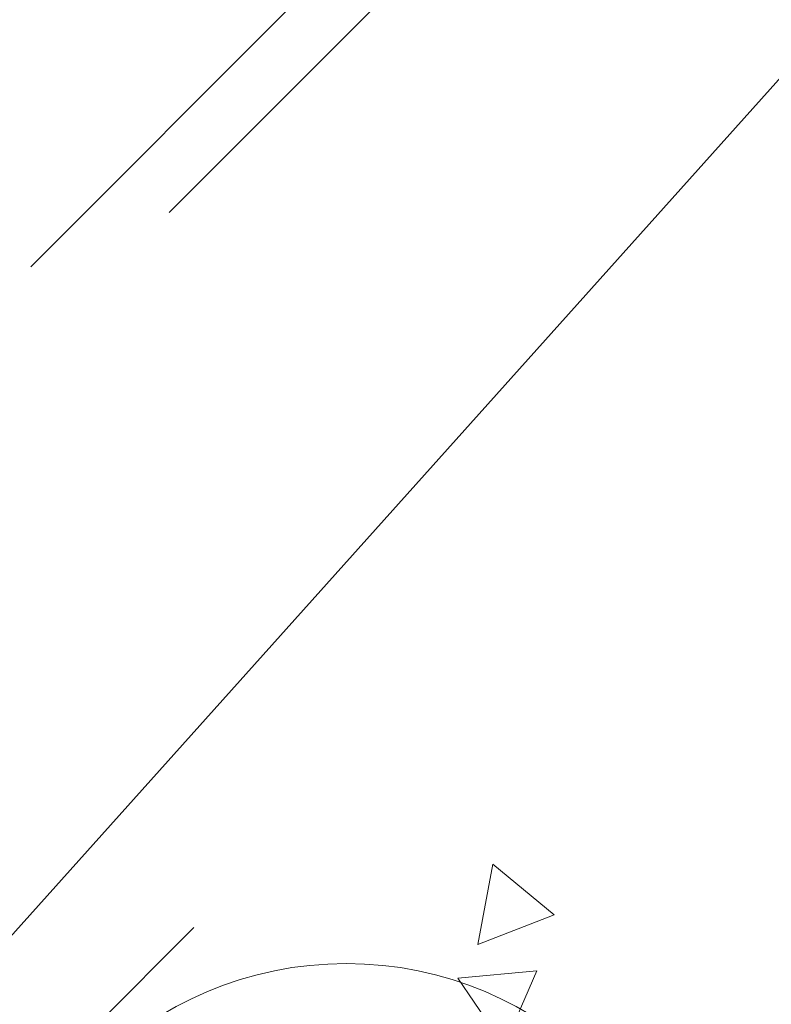
# Model space of a CAD drawing. Units: inches. Extents: x 375 to 1122, y 27 to 1069.
# Tile 124 of 155: x 720.77 to 731.16, y 886.61 to 900.21. Entities that reach past the tile are written whole.
import ezdxf

# ---------------------------------------------------------------- set-up
doc = ezdxf.new("R2010")
doc.units = ezdxf.units.IN
doc.layers.add('A-ANNO-DIMS', color=2, linetype='Continuous', lineweight=18)
doc.layers.add('Furniture', color=30, linetype='Continuous', lineweight=18)
doc.styles.get("Standard").update_dxf_attribs({"font": 'arial.ttf'})
doc.dimstyles.new('ISO-25', dxfattribs={"dimtxt": 12, "dimasz": 2.5, "dimexe": 1.5, "dimexo": 1.5, "dimtad": 1, "dimdec": 1, "dimlunit": 3, "dimtxsty": 'Standard', "dimblk": 'ARCHTICK', "dimcen": 2.5, "dimadec": 0, "dimazin": 0, "dimtfac": 1, "dimtdec": 1, "dimtmove": 0, "dimatfit": 3, "dimfxl": 1.5, "dimfxlon": 1, "dimarcsym": 0})

# ---------------------------------------------------------------- blocks, each defined once
blk = doc.blocks.new('A$C403C54AD')
for p, q in [((0.95931, 1.17062, -0.0006), (1.35847, 0.81256, -0.0006)), ((1.24444, 1.05916, -0.0006), (1.26195, 1.08031, -0.0006)), ((1.26195, 1.08031, -0.0006), (1.27222, 1.05396, -0.0006)), ((1.28381, 1.04703, -0.0006), (1.28124, 1.07437, -0.0006)), ((1.28124, 1.07437, -0.0006), (1.30713, 1.06299, -0.0006)), ((1.30713, 1.06299, -0.0006), (1.28381, 1.04703, -0.0006)), ((0.90685, 1.05977, -0.0006), (1.01943, 0.94723, -0.0006)), ((1.27222, 1.05396, -0.0006), (1.24444, 1.05916, -0.0006)), ((0.92556, 1.01193, -0.0006), (1.03814, 0.8994, -0.0006)), ((1.26636, 0.95578, -0.0006), (1.37894, 0.84325, -0.0006))]:
    blk.add_line(p, q)
blk.add_circle((1.40208, 1.00844, -0.0006), 0.12331)
blk = doc.blocks.new('_ArchTick')
at = {"color": 0, "linetype": 'ByBlock', "const_width": 0.15}
blk.add_lwpolyline([(-0.5, -0.5), (0.5, 0.5)], dxfattribs=at)
blk = doc.blocks.new('*D73')
at = {"layer": 'A-ANNO-DIMS', "color": 0, "lineweight": -2, "transparency": 16777216}
for p, q in [((686.757, 932.428), (686.757, 929.428)), ((770.757, 932.428), (770.757, 929.428)), ((686.757, 930.928), (770.757, 930.928)), ((770.757, 930.928), (987.61, 930.928))]:
    blk.add_line(p, q, dxfattribs=at)
at = {"layer": 'Defpoints', "color": 0, "transparency": 16777216}
for p in [(686.757, 943.528), (770.757, 943.528), (770.757, 930.928)]:
    blk.add_point(p, dxfattribs=at)
at = {"layer": 'A-ANNO-DIMS', "color": 0, "lineweight": -2, "transparency": 16777216, "xscale": 2.5, "yscale": 2.5, "zscale": 2.5, "rotation": 180}
blk.add_blockref('_ArchTick', (686.757, 930.928), dxfattribs=at)
at = {"layer": 'A-ANNO-DIMS', "color": 0, "lineweight": -2, "transparency": 16777216, "xscale": 2.5, "yscale": 2.5, "zscale": 2.5}
blk.add_blockref('_ArchTick', (770.757, 930.928), dxfattribs=at)
at = {"layer": 'A-ANNO-DIMS', "color": 0, "transparency": 16777216, "insert": (880.433, 937.757), "char_height": 12, "attachment_point": 5}
blk.add_mtext('2-PANEL SLIDER 7\'-0" TYP.', dxfattribs=at)
blk = doc.blocks.new('*D88')
at = {"layer": 'A-ANNO-DIMS', "color": 0, "lineweight": -2, "transparency": 16777216}
for p, q in [((731.007, 1052.528), (731.007, 1055.528)), ((854.007, 1052.528), (854.007, 1055.528)), ((731.007, 1054.028), (854.007, 1054.028))]:
    blk.add_line(p, q, dxfattribs=at)
at = {"layer": 'Defpoints', "color": 0, "transparency": 16777216}
for p in [(854.007, 1054.028), (731.007, 502.528), (854.007, 502.528)]:
    blk.add_point(p, dxfattribs=at)
at = {"layer": 'A-ANNO-DIMS', "color": 0, "lineweight": -2, "transparency": 16777216, "xscale": 2.5, "yscale": 2.5, "zscale": 2.5, "rotation": 180}
blk.add_blockref('_ArchTick', (731.007, 1054.028), dxfattribs=at)
at = {"layer": 'A-ANNO-DIMS', "color": 0, "lineweight": -2, "transparency": 16777216, "xscale": 2.5, "yscale": 2.5, "zscale": 2.5}
blk.add_blockref('_ArchTick', (854.007, 1054.028), dxfattribs=at)
at = {"layer": 'A-ANNO-DIMS', "color": 0, "transparency": 16777216, "insert": (792.507, 1060.784), "char_height": 12, "attachment_point": 5}
blk.add_mtext('10\'-3"', dxfattribs=at)
blk = doc.blocks.new('*D91')
at = {"layer": 'A-ANNO-DIMS', "color": 0, "lineweight": -2, "transparency": 16777216}
for p, q in [((728.007, 1052.528), (728.007, 1055.528)), ((788.007, 1052.528), (788.007, 1055.528)), ((728.007, 1054.028), (788.007, 1054.028))]:
    blk.add_line(p, q, dxfattribs=at)
at = {"layer": 'Defpoints', "color": 0, "transparency": 16777216}
for p in [(788.007, 1054.028), (728.007, 774.028), (788.007, 774.028)]:
    blk.add_point(p, dxfattribs=at)
at = {"layer": 'A-ANNO-DIMS', "color": 0, "lineweight": -2, "transparency": 16777216, "xscale": 2.5, "yscale": 2.5, "zscale": 2.5, "rotation": 180}
blk.add_blockref('_ArchTick', (728.007, 1054.028), dxfattribs=at)
at = {"layer": 'A-ANNO-DIMS', "color": 0, "lineweight": -2, "transparency": 16777216, "xscale": 2.5, "yscale": 2.5, "zscale": 2.5}
blk.add_blockref('_ArchTick', (788.007, 1054.028), dxfattribs=at)
at = {"layer": 'A-ANNO-DIMS', "color": 0, "transparency": 16777216, "insert": (758.007, 1060.78), "char_height": 12, "attachment_point": 5}
blk.add_mtext('5\'-0"', dxfattribs=at)

msp = doc.modelspace()

# ---------------------------------------------------------------- block references
at = {"layer": 'Furniture', "xscale": 39.9918517141215, "yscale": 39.9918517141215, "zscale": 39.9918517141215, "rotation": 270}
msp.add_blockref('A$C403C54AD', (684.955, 938.316, 0.024), dxfattribs=at)

# ---------------------------------------------------------------- dimensions: what is measured, and where the dimension line sits
at = {"layer": 'A-ANNO-DIMS'}
for base, p1, p2, picture, middle in [((788.007, 1054.028), (728.007, 774.028), (788.007, 774.028), '*D91', (758.007, 1060.78)), ((854.007, 1054.028), (731.007, 502.528), (854.007, 502.528), '*D88', (792.507, 1060.784))]:
    dim = msp.add_linear_dim(base=base, p1=p1, p2=p2, dimstyle='ISO-25', override={"dimdec": 1, "dimlfac": 1, "dimrnd": 0, "dimzin": 1, "dimdsep": 46, "dimlunit": 4, "dimfrac": 2}, dxfattribs=at)
    dim.commit()
    dim.dimension.update_dxf_attribs({"geometry": picture, "text_midpoint": middle})
dim = msp.add_linear_dim(base=(770.757, 930.928), p1=(686.757, 943.528), p2=(770.757, 943.528), text='2-PANEL SLIDER <> TYP.', dimstyle='ISO-25', override={"dimdec": 1, "dimlfac": 1, "dimrnd": 0, "dimzin": 1, "dimdsep": 46, "dimlunit": 4, "dimfrac": 2}, dxfattribs=at)
dim.commit()
dim.dimension.update_dxf_attribs({"geometry": '*D73', "text_midpoint": (880.433, 937.757)})

doc.saveas('drawing.dxf')
